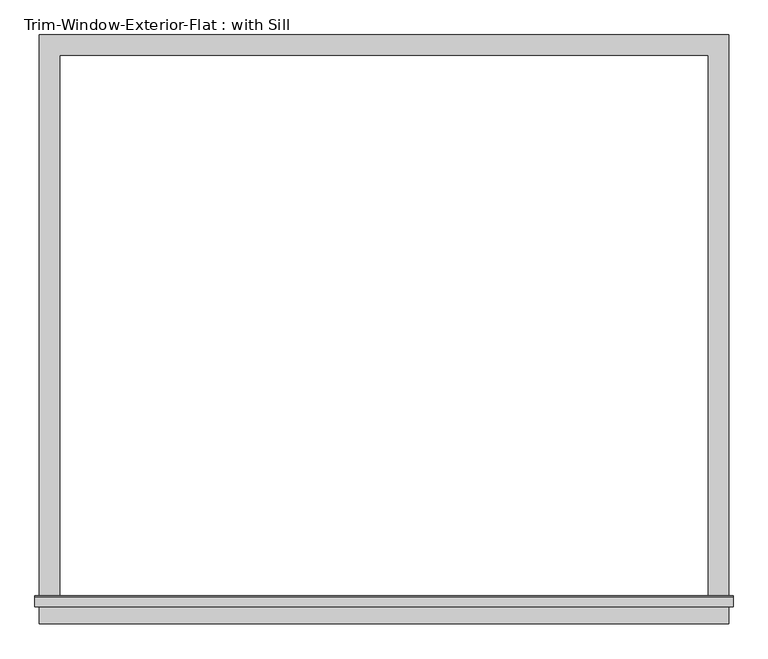
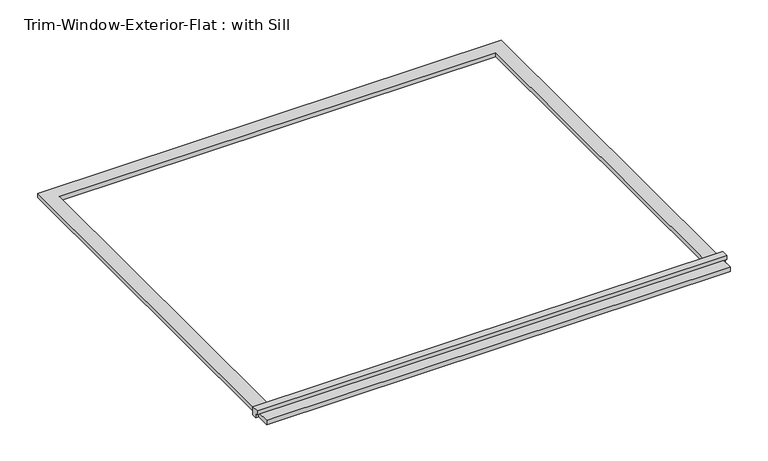
"""IFC4 building model written with IfcOpenShell, lengths in millimetres: proxy geometry, Trim-Window-Exterior-Flat : with Sill."""

from ifc_helpers import new_model, si_unit, frame, origin, origin_with_axes, place, context, project, spatial, polyline, outline, extrude, source, transform, mapped, element, save


def trim_window_exterior_flat_with_sill_c22f0c79(model_context):
    return source(origin(), model_context, "Body", "SweptSolid", [
        extrude(outline(polyline([(971.55, -1546.1823709), (971.55, -1603.3323709), (-971.55, -1603.3323709), (-971.55, -1546.1823709), (971.55, -1546.1823709)])), origin_with_axes(), (0.0, 0.0, 1.0), 19.05),
        extrude(outline(polyline([(-1555.75, 38.1), (-1526.4580645, 38.1), (-1524.0, 19.05), (-1524.0, 0.0), (-1546.1823709, 0.0), (-1546.1823709, 19.05), (-1555.75, 19.05), (-1555.75, 38.1)])), frame((-984.25, 0.0, 0.0), z_axis=(1.0, 0.0, 0.0), x_axis=(0.0, 1.0, 0.0)), (0.0, 0.0, 1.0), 1968.5),
        extrude(outline(polyline([(-971.55, 57.15), (971.55, 57.15), (971.55, -1524.0), (914.4, -1524.0), (914.4, 0.0), (-914.4, 0.0), (-914.4, -1524.0), (-971.55, -1524.0), (-971.55, 57.15)])), origin_with_axes(), (0.0, 0.0, 1.0), 19.05),
    ])


if __name__ == "__main__":
    model = new_model("IFC4")
    model_context = context("Model", 3, world=origin())
    ifc_project = project(units=[si_unit("LENGTHUNIT", "METRE", prefix="MILLI")], contexts=[model_context])
    site = spatial("IfcSite", under=ifc_project)
    building = spatial("IfcBuilding", under=site)
    placement = place(None, origin())
    trim_window_exterior_flat_with_sill_shape = trim_window_exterior_flat_with_sill_c22f0c79(model_context)
    element("IfcBuildingElementProxy", 1, Name="Trim-Window-Exterior-Flat : with Sill", ObjectType="Trim-Window-Exterior-Flat : with Sill", at=placement, inside=building, context=model_context, shape_type="MappedRepresentation", body=[
        mapped(trim_window_exterior_flat_with_sill_shape, transform((0.0, 0.0, 0.0), x_axis=(1.0, 0.0, 0.0), y_axis=(0.0, 1.0, 0.0), z_axis=(0.0, 0.0, 1.0))),
    ])
    save(model, "model.ifc")

# Revit data of these elements
# Type "Trim-Window-Exterior-Flat : with Sill"
#   Trim Width = 0' - 2 1/4"
#   Trim Thickness_Picture Frame = 0' - 1 1/4"
#   Trim Thickness_with Sill = 0' - 0 3/4"
#   Sill Thickness = 0' - 1 1/4"
#   Opening Width [instance default] = 2' - 0"
#   Opening Height [instance default] = 3' - 0"
#   Default Elevation = 4' - 0"
#   Sill = yes
#   Picture Frame = no
#   Trim Material [instance default] = none
# Element 1 (IfcBuildingElementProxy, "Trim-Window-Exterior-Flat : with Sill")
#   Opening Width = 6' - 0"
#   Opening Height = 5' - 0"
#   Trim Material = Clad - White
#   Materials on its faces: "Clad - White"
# Materials
#   "Clad - White": class "Wood", colour RGB 242 242 238, transparency 0, Cost = 0
